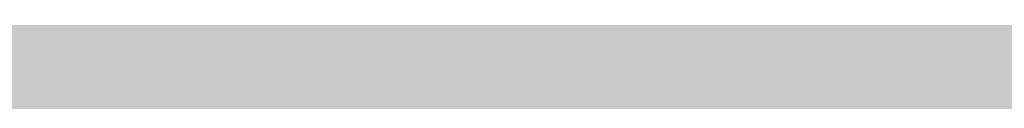
# Model space of a CAD drawing. Units: feet. Extents: x 3168 to 4724, y 827 to 1477.
# Tile 185 of 256: x 3307.378 to 3316.072, y 1098.344 to 1099.001. Entities that reach past the tile are written whole.
import ezdxf

# ---------------------------------------------------------------- set-up
doc = ezdxf.new("R2010")
doc.units = ezdxf.units.FT
doc.layers.add('A-ELEV', color=7, linetype='Continuous', lineweight=35)
doc.layers.add('A-ELEV-PATT', color=8, linetype='Continuous', lineweight=13)

msp = doc.modelspace()

# ---------------------------------------------------------------- hatches: boundary and pattern name
at = {"layer": 'A-ELEV-PATT'}
h = msp.add_hatch(color=256, dxfattribs=at)
h.dxf.hatch_style = 1
edge = h.paths.add_edge_path()
edge.add_ellipse((3552.9058, 979.2201), major_axis=(36.7449, 0), ratio=0.4848485, start_angle=0, end_angle=360)
edge = h.paths.add_edge_path()
edge.add_ellipse((3559.8916, 929.2523), major_axis=(36.7449, 0), ratio=0.4848485, start_angle=0, end_angle=360)
edge = h.paths.add_edge_path()
edge.add_line((3299.3168, 1198.6061), (3479.9167, 1198.6061))
edge.add_line((3479.9167, 1198.6061), (3479.9167, 1209.8686))
edge.add_spline(control_points=[(3479.9167, 1209.8686), (3464.3012, 1209.8686), (3448.6856, 1209.8686), (3410.9491, 1209.8686), (3388.8282, 1209.8686), (3355.6469, 1209.8686), (3344.5864, 1209.8686), (3327.9957, 1209.8686), (3322.4655, 1209.8686), (3314.1702, 1209.8686), (3311.4051, 1209.8686), (3307.2574, 1209.8686), (3305.8748, 1209.8686), (3303.801, 1209.8686), (3303.1097, 1209.8686), (3302.0728, 1209.8686), (3301.7272, 1209.8686), (3301.2087, 1209.8686), (3301.0359, 1209.8686), (3300.7767, 1209.8686), (3300.6903, 1209.8686), (3300.5606, 1209.8686), (3300.5174, 1209.8686), (3300.4526, 1209.8686), (3300.431, 1209.8686), (3300.3986, 1209.8686), (3300.3878, 1209.8686), (3300.3662, 1209.8686), (3300.3457, 1209.8686), (3300.3455, 1209.8686), (3300.3455, 1209.8686), (3300.3433, 1209.8686), (3300.3411, 1209.8686), (3300.3379, 1209.8686), (3300.3368, 1209.8686), (3300.3339, 1209.8686), (3300.3321, 1209.8686), (3300.3255, 1209.8686), (3300.3207, 1209.8686), (3300.3109, 1209.8686), (3300.306, 1209.8686), (3300.2905, 1209.8686), (3300.28, 1209.8686), (3300.2324, 1209.8688), (3300.1953, 1209.869), (3299.9511, 1209.8706), (3299.7448, 1209.8743), (3299.4368, 1209.8833), (3299.3344, 1209.8868), (3299.1811, 1209.8929), (3299.13, 1209.8951), (3298.6522, 1209.9168), (3298.2295, 1209.9457), (3297.6016, 1210.0024), (3297.3934, 1210.0235), (3297.0827, 1210.0583), (3296.9793, 1210.0705), (3296.293, 1210.1549), (3295.7181, 1210.2434), (3294.8687, 1210.3989), (3294.5877, 1210.4545), (3294.1693, 1210.5433), (3294.0304, 1210.5739), (3291.7071, 1211.1012), (3289.6536, 1211.8134), (3285.7763, 1213.564), (3283.9514, 1214.6035), (3280.5122, 1216.9801), (3278.8972, 1218.3176), (3276.3799, 1220.8295), (3275.416, 1221.9177), (3274.0393, 1223.7077), (3273.581, 1224.3495), (3273.1432, 1225.0163)], knot_values=[39.119033, 39.119033, 39.119033, 39.119033, 39.286353, 39.286353, 39.523379, 39.523379, 39.641892, 39.641892, 39.701148, 39.701148, 39.730777, 39.730777, 39.745591, 39.745591, 39.752998, 39.752998, 39.756701, 39.756701, 39.758553, 39.758553, 39.759479, 39.759479, 39.759942, 39.759942, 39.760173, 39.760173, 39.760289, 39.760289, 39.760405, 39.760405, 39.760463, 39.760463, 39.763389, 39.763389, 39.764851, 39.764851, 39.767304, 39.767304, 39.773825, 39.773825, 39.78057, 39.78057, 39.79477, 39.79477, 39.845194, 39.845194, 40.126715, 40.126715, 40.267476, 40.267476, 40.337856, 40.337856, 40.927023, 40.927023, 41.221606, 41.221606, 41.368898, 41.368898, 42.202622, 42.202622, 42.619485, 42.619485, 42.827916, 42.827916, 46.118323, 46.118323, 49.408731, 49.408731, 52.699139, 52.699139, 54.927489, 54.927489, 56.104228, 56.104228, 56.104228, 56.104228], weights=[1, 1, 1, 1, 1, 1, 1, 1, 1, 1, 1, 1, 1, 1, 1, 1, 1, 1, 1, 1, 1, 1, 1, 1, 1, 1, 1, 1, 1, 1, 1, 1, 1, 1, 1, 1, 1, 1, 1, 1, 1, 1, 1, 1, 1, 1, 1, 1, 1, 1, 1, 1, 1, 1, 1, 1, 1, 1, 1, 1, 1, 1, 1, 1, 1, 1, 1, 1, 1, 1, 1, 1, 1, 1], degree=3, periodic=0)
edge.add_line((3273.1432, 1225.0163), (3273.1432, 1099.0163))
edge.add_line((3273.1432, 1099.0163), (3299.3168, 1099.0163))
edge.add_line((3299.3168, 1099.0163), (3299.3168, 1198.6061))
edge = h.paths.add_edge_path()
edge.add_line((3304.7584, 1324.1581), (3479.9167, 1324.1581))
edge.add_line((3479.9167, 1324.1581), (3479.9167, 1335.7146))
edge.add_line((3479.9167, 1335.7146), (3269.1616, 1335.7146))
edge.add_spline(control_points=[(3269.1616, 1335.7146), (3264.0242, 1335.7146), (3258.3641, 1328.9582), (3259.2643, 1323.9003)], knot_values=[0, 0, 0, 0, 15.412191, 15.412191, 15.412191, 15.412191], degree=3, periodic=0)
edge.add_line((3259.2643, 1323.9003), (3265.5168, 1288.7691))
edge.add_line((3265.5168, 1288.7691), (3275.2651, 1261.5456))
edge.add_line((3275.2651, 1261.5456), (3304.7584, 1261.5456))
edge.add_line((3304.7584, 1261.5456), (3304.7584, 1324.1581))
h = msp.add_hatch(color=256, dxfattribs=at)
h.dxf.hatch_style = 1
h.paths.add_polyline_path([(3384.5252, 1099.0163), (3335.0292, 1099.0163), (3299.3168, 1099.0163), (3273.1432, 1099.0163), (3217.5654, 1099.0163), (3168.0693, 827.1163), (3335.0292, 827.1163)])

# ---------------------------------------------------------------- linework, layer by layer
at = {"layer": 'A-ELEV'}
msp.add_open_spline([(3808.5202, 1099.0163), (3808.5202, 1141.4132), (3808.5202, 1183.8102), (3808.5202, 1226.6353), (3808.5202, 1227.0636), (3808.5202, 1227.4918), (3811.4919, 1248.9947), (3814.4635, 1270.4975), (3817.4652, 1292.2176), (3817.4952, 1292.4348), (3817.5253, 1292.652), (3817.5728, 1310.1067), (3817.6203, 1327.5615), (3817.6679, 1345.0163), (3817.6679, 1345.458), (3817.6679, 1345.8996), (3817.6679, 1346.456), (3817.6679, 1346.5708), (3817.6679, 1346.7529), (3817.6679, 1346.8201), (3817.6679, 1346.9349), (3817.6679, 1346.9823), (3817.6679, 1347.0386), (3817.6679, 1347.0474), (3817.6679, 1347.0737), (3817.6679, 1347.0593), (3817.6679, 1347.0615), (3817.6679, 1347.0627), (3817.6679, 1347.066), (3817.6679, 1347.0683), (3817.6679, 1347.075), (3817.6679, 1347.0795), (3817.6678, 1347.0929), (3817.6678, 1347.1019), (3817.6678, 1347.1288), (3817.6677, 1347.1467), (3817.6674, 1347.2004), (3817.6672, 1347.2362), (3817.6661, 1347.3434), (3817.665, 1347.4147), (3817.6608, 1347.6281), (3817.6566, 1347.7697), (3817.64, 1348.1925), (3817.6235, 1348.4716), (3817.5591, 1349.3001), (3817.4961, 1349.8406), (3817.2554, 1351.4242), (3817.0263, 1352.4288), (3816.3069, 1354.8889), (3815.7437, 1356.2687), (3814.464, 1358.8192), (3813.7464, 1359.991), (3812.1958, 1362.1723), (3811.3622, 1363.1821), (3809.5888, 1365.069), (3808.6488, 1365.9461), (3806.6543, 1367.5796), (3805.5997, 1368.3362), (3803.3529, 1369.7223), (3802.1605, 1370.3524), (3799.6008, 1371.4536), (3798.2327, 1371.9255), (3795.2801, 1372.6346), (3793.6931, 1372.8721), (3791.8694, 1372.9265), (3791.7409, 1372.9292), (3791.3534, 1372.9341), (3791.0927, 1372.9329), (3790.3041, 1372.9151), (3789.7695, 1372.8842), (3789.2092, 1372.8302), (3789.1906, 1372.8284), (3789.1349, 1372.8229), (3789.0977, 1372.8191), (3789.0484, 1372.814), (3789.0364, 1372.8127), (3789.0003, 1372.8089), (3788.9761, 1372.8063), (3788.9494, 1372.8034), (3788.9468, 1372.8031), (3788.9426, 1372.8027), (3788.941, 1372.8025), (3788.9386, 1372.8022), (3788.9378, 1372.8021), (3788.9354, 1372.8019), (3788.8675, 1372.7944), (3788.7569, 1372.7822), (3788.7015, 1372.7761), (3788.5355, 1372.7579), (3788.4249, 1372.7457), (3788.0929, 1372.7092), (3787.8715, 1372.6848), (3787.2075, 1372.6118), (3786.7648, 1372.5631), (3785.4368, 1372.417), (3784.5515, 1372.3196), (3781.8954, 1372.0274), (3780.1247, 1371.8327), (3774.8126, 1371.2483), (3771.2713, 1370.8587), (3760.6471, 1369.69), (3753.5643, 1368.9109), (3732.316, 1366.5735), (3718.1504, 1365.0152), (3694.0068, 1362.3593), (3684.0287, 1361.2617), (3674.0506, 1360.1641), (3664.6007, 1360.1641), (3655.1508, 1360.1641), (3626.8011, 1360.1641), (3607.9013, 1360.1641), (3551.2019, 1360.1641), (3513.4023, 1360.1641), (3467.7252, 1360.1641), (3459.8476, 1360.1641), (3436.2149, 1360.1641), (3420.4597, 1360.1641), (3373.1943, 1360.1641), (3341.6839, 1360.1641), (3302.8482, 1360.1641), (3295.5227, 1360.1641), (3286.0383, 1360.1641), (3283.8794, 1360.1641), (3277.4026, 1360.1641), (3273.0848, 1360.1641), (3267.7329, 1360.1641), (3266.6988, 1360.1641), (3263.5965, 1360.1641), (3261.5284, 1360.1641), (3259.2369, 1360.1641), (3259.0137, 1360.1641), (3258.344, 1360.1641), (3257.8975, 1360.1641), (3257.431, 1360.1641), (3257.411, 1360.1641), (3257.3706, 1360.1641), (3257.3755, 1360.1641), (3257.3746, 1360.1641), (3257.3739, 1360.1641), (3257.372, 1360.1641), (3257.3706, 1360.1641), (3257.3667, 1360.1641), (3257.364, 1360.1641), (3257.3561, 1360.1641), (3257.3508, 1360.164), (3257.335, 1360.164), (3257.3244, 1360.164), (3257.2928, 1360.1639), (3257.2717, 1360.1638), (3257.2084, 1360.1634), (3257.1663, 1360.163), (3257.0402, 1360.1614), (3256.9563, 1360.1598), (3256.7055, 1360.1534), (3256.5392, 1360.147), (3256.0436, 1360.1219), (3255.7173, 1360.0971), (3254.7524, 1360.0005), (3254.128, 1359.9065), (3252.1801, 1359.5253), (3250.9416, 1359.144), (3248.6702, 1358.2433), (3247.6357, 1357.7238), (3245.7326, 1356.6035), (3244.8634, 1356.0021), (3243.2531, 1354.7429), (3242.512, 1354.0847), (3240.7511, 1352.3448), (3239.801, 1351.2296), (3238.0878, 1348.8724), (3237.3247, 1347.6304), (3235.9825, 1344.9716), (3235.4022, 1343.5549), (3234.5911, 1340.8155), (3234.3109, 1339.5435), (3233.9765, 1336.8026), (3233.9221, 1335.3309), (3234.1489, 1332.5913), (3234.3495, 1331.3672), (3234.7199, 1329.9994), (3234.7524, 1329.8834), (3234.8536, 1329.5348), (3234.9259, 1329.3017), (3235.0248, 1329.0026), (3235.0469, 1328.9369), (3235.0776, 1328.8472), (3235.0859, 1328.8232), (3235.1109, 1328.7511), (3235.1278, 1328.703), (3235.148, 1328.6462), (3235.1511, 1328.6376), (3235.1561, 1328.6235), (3235.1581, 1328.618), (3235.1602, 1328.612), (3235.1656, 1328.5969), (3235.1801, 1328.5565), (3235.1903, 1328.5281), (3235.2208, 1328.4429), (3235.2411, 1328.3862), (3235.3021, 1328.2159), (3235.3427, 1328.1023), (3235.4647, 1327.7617), (3235.546, 1327.5346), (3235.79, 1326.8534), (3235.9526, 1326.3992), (3236.4405, 1325.0367), (3236.7657, 1324.1284), (3237.7415, 1321.4034), (3238.392, 1319.5868), (3240.3435, 1314.1369), (3241.6445, 1310.5036), (3245.5476, 1299.6037), (3248.1496, 1292.3371), (3255.9557, 1270.5374), (3261.1598, 1256.0042), (3267.3876, 1238.612), (3268.4114, 1235.7529), (3269.5104, 1232.6839), (3269.5856, 1232.4739), (3269.7066, 1232.1359), (3269.7524, 1232.0079), (3269.8273, 1231.7987), (3269.8564, 1231.7176), (3269.9063, 1231.5781), (3269.9272, 1231.5198), (3269.9725, 1231.3934), (3269.9968, 1231.3254), (3270.0265, 1231.2425), (3270.0318, 1231.2277), (3270.0403, 1231.204), (3270.0392, 1231.207), (3270.0394, 1231.2066), (3270.0394, 1231.2064), (3270.0396, 1231.2058), (3270.0398, 1231.2055), (3270.0402, 1231.2043), (3270.0404, 1231.2036), (3270.0413, 1231.2013), (3270.0418, 1231.1998), (3270.0434, 1231.1953), (3270.0445, 1231.1922), (3270.0478, 1231.1832), (3270.0499, 1231.1771), (3270.0564, 1231.159), (3270.0608, 1231.147), (3270.0739, 1231.1108), (3270.0826, 1231.0867), (3270.1089, 1231.0144), (3270.1266, 1230.9663), (3270.1799, 1230.8225), (3270.2159, 1230.7269), (3270.3253, 1230.4415), (3270.4, 1230.2528), (3270.6292, 1229.6914), (3270.7889, 1229.3235), (3271.2865, 1228.2383), (3271.6431, 1227.5398), (3272.7759, 1225.5153), (3273.6142, 1224.2605), (3275.416, 1221.9177), (3276.3799, 1220.8295), (3278.8972, 1218.3176), (3280.5122, 1216.9801), (3283.9514, 1214.6035), (3285.7763, 1213.564), (3289.6536, 1211.8134), (3291.7071, 1211.1012), (3294.0304, 1210.5739), (3294.1693, 1210.5433), (3294.5877, 1210.4545), (3294.8687, 1210.3989), (3295.7181, 1210.2434), (3296.293, 1210.1549), (3296.9793, 1210.0705), (3297.0827, 1210.0583), (3297.3934, 1210.0235), (3297.6016, 1210.0024), (3298.2295, 1209.9457), (3298.6522, 1209.9168), (3299.13, 1209.8951), (3299.1811, 1209.8929), (3299.3344, 1209.8868), (3299.4368, 1209.8833), (3299.7448, 1209.8743), (3299.9511, 1209.8706), (3300.1953, 1209.869), (3300.2324, 1209.8688), (3300.28, 1209.8686), (3300.2905, 1209.8686), (3300.306, 1209.8686), (3300.3109, 1209.8686), (3300.3207, 1209.8686), (3300.3255, 1209.8686), (3300.3321, 1209.8686), (3300.3339, 1209.8686), (3300.3368, 1209.8686), (3300.3379, 1209.8686), (3300.3411, 1209.8686), (3300.3433, 1209.8686), (3300.3455, 1209.8686), (3300.3455, 1209.8686), (3300.3457, 1209.8686), (3300.3662, 1209.8686), (3300.3878, 1209.8686), (3300.3986, 1209.8686), (3300.431, 1209.8686), (3300.4526, 1209.8686), (3300.5174, 1209.8686), (3300.5606, 1209.8686), (3300.6903, 1209.8686), (3300.7767, 1209.8686), (3301.0359, 1209.8686), (3301.2087, 1209.8686), (3301.7272, 1209.8686), (3302.0728, 1209.8686), (3303.1097, 1209.8686), (3303.801, 1209.8686), (3305.8748, 1209.8686), (3307.2574, 1209.8686), (3311.4051, 1209.8686), (3314.1702, 1209.8686), (3322.4655, 1209.8686), (3327.9957, 1209.8686), (3344.5864, 1209.8686), (3355.6469, 1209.8686), (3388.8282, 1209.8686), (3410.9491, 1209.8686), (3477.3119, 1209.8686), (3521.5537, 1209.8686), (3566.8362, 1209.8686), (3567.8769, 1209.8686), (3570.999, 1209.8686), (3573.0804, 1209.8686), (3575.7814, 1209.8686), (3576.4009, 1209.8686), (3577.2958, 1209.8686), (3577.5712, 1209.8686), (3578.3971, 1209.8686), (3578.9478, 1209.8686), (3579.7565, 1209.8686), (3580.0145, 1209.8686), (3580.3427, 1209.8686), (3580.3269, 1209.8686), (3580.3272, 1209.8686), (3580.3273, 1209.8686), (3580.3278, 1209.8686), (3580.3281, 1209.8686), (3580.329, 1209.8686), (3580.3296, 1209.8686), (3580.3314, 1209.8686), (3580.3327, 1209.8686), (3580.3363, 1209.8686), (3580.3388, 1209.8686), (3580.3461, 1209.8686), (3580.351, 1209.8686), (3580.3657, 1209.8685), (3580.3754, 1209.8685), (3580.4048, 1209.8684), (3580.4244, 1209.8684), (3580.4832, 1209.8681), (3580.5224, 1209.8678), (3580.6404, 1209.8666), (3580.7192, 1209.8655), (3580.9563, 1209.8608), (3581.1152, 1209.8561), (3581.5942, 1209.8372), (3581.9164, 1209.8183), (3582.8899, 1209.7424), (3583.548, 1209.6662), (3585.5318, 1209.3606), (3586.8672, 1209.0539), (3589.4715, 1208.2525), (3590.7402, 1207.7579), (3591.9955, 1207.1588), (3592.0578, 1207.1287), (3592.2442, 1207.038), (3592.3677, 1206.9766), (3592.7353, 1206.7904), (3592.9768, 1206.6631), (3593.2445, 1206.5164), (3593.2747, 1206.4998), (3593.3651, 1206.4498), (3593.4251, 1206.4163), (3593.6043, 1206.3153), (3593.7227, 1206.2472), (3593.8572, 1206.1684), (3593.8744, 1206.1583), (3593.9257, 1206.128), (3593.9599, 1206.1078), (3594.0621, 1206.0469), (3594.1298, 1206.0061), (3594.2084, 1205.9582), (3594.2197, 1205.9513), (3594.2534, 1205.9307), (3594.2758, 1205.9169), (3594.343, 1205.8755), (3594.3876, 1205.8479), (3594.4336, 1205.819), (3594.4353, 1205.818), (3594.4402, 1205.8149), (3594.4435, 1205.8129), (3594.4471, 1205.8106), (3594.4475, 1205.8103), (3594.4487, 1205.8096), (3594.4495, 1205.8091), (3594.4504, 1205.8086), (3594.4505, 1205.8085), (3594.4506, 1205.8084), (3594.4674, 1205.7979), (3594.4933, 1205.7817), (3594.5062, 1205.7736), (3594.545, 1205.7492), (3594.5709, 1205.733), (3594.6485, 1205.6844), (3594.7002, 1205.652), (3594.8554, 1205.5547), (3594.9589, 1205.4898), (3595.2694, 1205.2953), (3595.4763, 1205.1656), (3596.0972, 1204.7765), (3596.5111, 1204.5171), (3597.7528, 1203.7388), (3598.5807, 1203.22), (3601.0642, 1201.6636), (3602.7198, 1200.6259), (3607.6868, 1197.513), (3610.9981, 1195.4377), (3620.932, 1189.2119), (3627.5546, 1185.0614), (3647.4225, 1172.6097), (3660.6678, 1164.3086), (3700.4035, 1139.4053), (3726.894, 1122.8031), (3757.2057, 1103.8061), (3761.027, 1101.4112), (3764.8482, 1099.0163), (3745.3283, 1099.0163), (3725.8083, 1099.0163), (3706.2884, 1099.0163), (3706.2884, 1108.4532), (3706.2884, 1117.8902), (3706.2884, 1127.3271), (3710.7508, 1127.3271), (3715.2131, 1127.3271), (3719.6755, 1127.3271)], degree=3, knots=[0, 0, 0, 0, 0.982037, 0.982037, 0.991957, 0.991957, 0.991957, 1.966522, 1.966522, 1.976367, 1.976367, 1.976367, 2.976367, 2.976367, 2.976367, 3.00169, 3.00169, 3.008272, 3.008272, 3.012129, 3.012129, 3.014851, 3.014851, 3.015353, 3.015353, 3.016359, 3.016359, 3.017365, 3.017365, 3.019376, 3.019376, 3.023398, 3.023398, 3.031442, 3.031442, 3.047531, 3.047531, 3.079708, 3.079708, 3.144063, 3.144063, 3.272772, 3.272772, 3.53019, 3.53019, 4.045026, 4.045026, 5.074698, 5.074698, 6.700878, 6.700878, 8.327058, 8.327058, 9.953238, 9.953238, 11.579418, 11.579418, 13.205598, 13.205598, 14.831778, 14.831778, 16.457958, 16.457958, 18.084138, 18.084138, 18.206872, 18.206872, 18.45234, 18.45234, 18.943275, 18.943275, 18.960093, 18.960093, 18.993729, 18.993729, 19.00461, 19.00461, 19.026374, 19.026374, 19.028737, 19.028737, 19.03018, 19.03018, 19.030897, 19.030897, 19.032332, 19.032332, 19.033766, 19.033766, 19.036636, 19.036636, 19.042374, 19.042374, 19.053851, 19.053851, 19.076805, 19.076805, 19.122714, 19.122714, 19.21453, 19.21453, 19.398163, 19.398163, 19.765429, 19.765429, 20.024128, 20.024128, 20.024128, 20.092031, 20.092031, 20.227836, 20.227836, 20.499446, 20.499446, 20.556051, 20.556051, 20.66926, 20.66926, 20.895678, 20.895678, 20.948316, 20.948316, 20.963829, 20.963829, 20.994855, 20.994855, 21.002285, 21.002285, 21.017146, 21.017146, 21.01875, 21.01875, 21.021959, 21.021959, 21.022102, 21.022102, 21.022249, 21.022249, 21.022708, 21.022708, 21.023627, 21.023627, 21.025464, 21.025464, 21.029138, 21.029138, 21.036486, 21.036486, 21.051183, 21.051183, 21.080575, 21.080575, 21.139361, 21.139361, 21.256932, 21.256932, 21.492073, 21.492073, 21.962356, 21.962356, 23.01002, 23.01002, 24.057684, 24.057684, 25.105348, 25.105348, 26.153011, 26.153011, 27.776787, 27.776787, 29.400562, 29.400562, 31.024337, 31.024337, 32.278801, 32.278801, 33.533265, 33.533265, 34.467568, 34.467568, 34.553971, 34.553971, 34.726776, 34.726776, 34.775309, 34.775309, 34.793079, 34.793079, 34.82862, 34.82862, 34.834979, 34.834979, 34.839039, 34.839039, 34.839411, 34.839411, 34.840285, 34.840285, 34.842034, 34.842034, 34.845531, 34.845531, 34.852525, 34.852525, 34.866512, 34.866512, 34.894488, 34.894488, 34.950439, 34.950439, 35.062342, 35.062342, 35.286147, 35.286147, 35.733758, 35.733758, 35.821815, 35.821815, 35.828283, 35.828283, 35.832225, 35.832225, 35.834724, 35.834724, 35.836521, 35.836521, 35.838617, 35.838617, 35.839073, 35.839073, 35.839345, 35.839345, 35.839617, 35.839617, 35.840161, 35.840161, 35.841249, 35.841249, 35.843425, 35.843425, 35.847778, 35.847778, 35.856482, 35.856482, 35.873891, 35.873891, 35.908709, 35.908709, 35.978345, 35.978345, 36.117617, 36.117617, 36.396161, 36.396161, 36.953248, 36.953248, 38.067423, 38.067423, 40.295772, 40.295772, 42.524122, 42.524122, 45.81453, 45.81453, 49.104937, 49.104937, 52.395345, 52.395345, 52.603776, 52.603776, 53.020639, 53.020639, 53.854363, 53.854363, 54.001655, 54.001655, 54.296238, 54.296238, 54.885405, 54.885405, 54.955785, 54.955785, 55.096546, 55.096546, 55.378067, 55.378067, 55.42849, 55.42849, 55.442691, 55.442691, 55.449436, 55.449436, 55.455957, 55.455957, 55.458409, 55.458409, 55.459872, 55.459872, 55.462798, 55.462798, 55.462856, 55.462856, 55.462972, 55.462972, 55.463088, 55.463088, 55.463319, 55.463319, 55.463782, 55.463782, 55.464708, 55.464708, 55.46656, 55.46656, 55.470263, 55.470263, 55.47767, 55.47767, 55.492484, 55.492484, 55.522112, 55.522112, 55.581369, 55.581369, 55.699882, 55.699882, 55.936907, 55.936907, 56.410959, 56.410959, 56.42211, 56.42211, 56.444413, 56.444413, 56.451051, 56.451051, 56.454001, 56.454001, 56.459901, 56.459901, 56.462666, 56.462666, 56.463418, 56.463418, 56.464171, 56.464171, 56.465675, 56.465675, 56.468684, 56.468684, 56.474702, 56.474702, 56.486738, 56.486738, 56.51081, 56.51081, 56.558955, 56.558955, 56.655243, 56.655243, 56.847821, 56.847821, 57.232975, 57.232975, 58.003284, 58.003284, 59.543901, 59.543901, 62.625137, 62.625137, 68.787607, 68.787607, 74.950078, 74.950078, 75.27336, 75.27336, 75.919923, 75.919923, 77.213051, 77.213051, 77.377769, 77.377769, 77.707206, 77.707206, 78.366079, 78.366079, 78.462532, 78.462532, 78.655436, 78.655436, 79.041245, 79.041245, 79.105735, 79.105735, 79.234714, 79.234714, 79.492672, 79.492672, 79.502197, 79.502197, 79.521249, 79.521249, 79.523534, 79.523534, 79.528103, 79.528103, 79.528682, 79.528682, 79.528885, 79.528885, 79.529089, 79.529089, 79.529495, 79.529495, 79.530308, 79.530308, 79.531935, 79.531935, 79.535187, 79.535187, 79.541693, 79.541693, 79.554704, 79.554704, 79.580725, 79.580725, 79.632769, 79.632769, 79.736856, 79.736856, 79.94503, 79.94503, 80.361377, 80.361377, 80.421435, 80.421435, 80.421435, 81.421435, 81.421435, 81.421435, 82.421435, 82.421435, 82.421435, 83.421435, 83.421435, 83.421435, 83.421435], dxfattribs=at)

doc.saveas('drawing.dxf')
